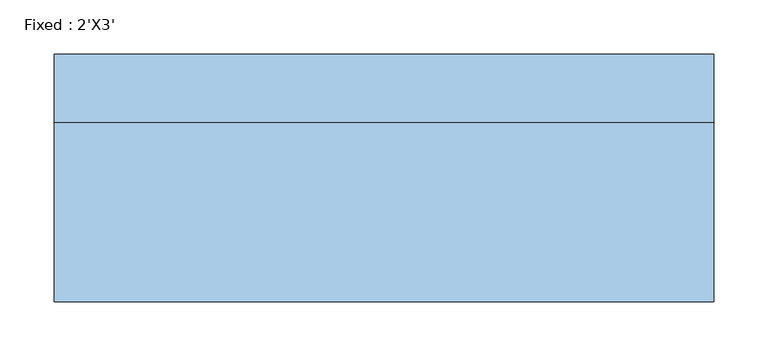
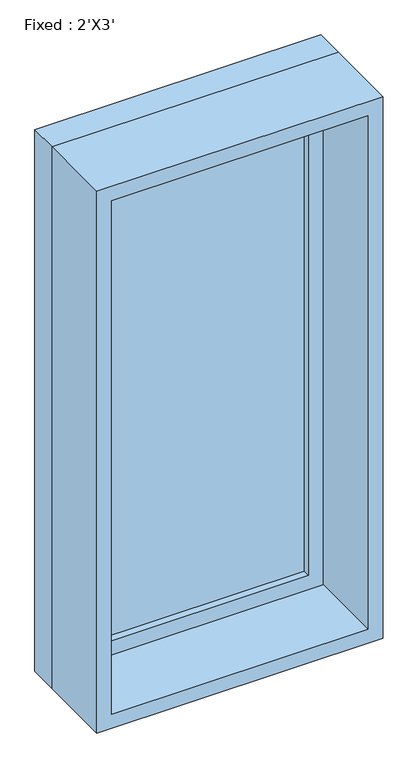
"""IFC4 building model written with IfcOpenShell, lengths in millimetres: window geometry, Fixed : 2'X3'."""

from ifc_helpers import new_model, si_unit, frame, origin, place, context, project, spatial, polyline, outline, extrude, source, transform, mapped, element, save


def fixed_2_x3_c82808a1(model_context):
    return source(origin(), model_context, "Body", "SweptSolid", [
        extrude(outline(polyline([(203.2, 66.675), (-279.4, 66.675), (-279.4, 79.375), (203.2, 79.375), (203.2, 66.675)])), frame((0.0, 0.0, 977.9), z_axis=(0.0, 0.0, 1.0), x_axis=(1.0, 0.0, 0.0)), (0.0, 0.0, 1.0), 1092.2),
        extrude(outline(polyline([(2114.55, -323.85), (933.45, -323.85), (933.45, 247.65), (2114.55, 247.65), (2114.55, -323.85)]), holes=[polyline([(2070.1, -279.4), (2070.1, 203.2), (977.9, 203.2), (977.9, -279.4), (2070.1, -279.4)])]), frame((0.0, 50.8, 0.0), z_axis=(0.0, 1.0, 0.0), x_axis=(0.0, 0.0, 1.0)), (0.0, 0.0, 1.0), 44.45),
        extrude(outline(polyline([(2133.6, -342.9), (914.4, -342.9), (914.4, 266.7), (2133.6, 266.7), (2133.6, -342.9)]), holes=[polyline([(2101.85, -311.15), (2101.85, 234.95), (946.15, 234.95), (946.15, -311.15), (2101.85, -311.15)])]), frame((0.0, -114.3, 0.0), z_axis=(0.0, 1.0, 0.0), x_axis=(0.0, 0.0, 1.0)), (0.0, 0.0, 1.0), 165.1),
        extrude(outline(polyline([(2133.6, 266.7), (2133.6, -342.9), (914.4, -342.9), (914.4, 266.7), (2133.6, 266.7)]), holes=[polyline([(2114.55, 247.65), (933.45, 247.65), (933.45, -323.85), (2114.55, -323.85), (2114.55, 247.65)])]), frame((0.0, 50.8, 0.0), z_axis=(0.0, 1.0, 0.0), x_axis=(0.0, 0.0, 1.0)), (0.0, 0.0, 1.0), 63.5),
    ])


if __name__ == "__main__":
    model = new_model("IFC4")
    model_context = context("Model", 3, world=origin())
    ifc_project = project(units=[si_unit("LENGTHUNIT", "METRE", prefix="MILLI")], contexts=[model_context])
    site = spatial("IfcSite", under=ifc_project)
    building = spatial("IfcBuilding", under=site)
    placement = place(None, origin())
    fixed_2_x3_shape = fixed_2_x3_c82808a1(model_context)
    element("IfcWindow", 1, ObjectType="Fixed : 2'X3'", at=placement, inside=building, context=model_context, shape_type="MappedRepresentation", body=[
        mapped(fixed_2_x3_shape, transform((0.0, 0.0, 0.0), x_axis=(1.0, 0.0, 0.0), y_axis=(0.0, 1.0, 0.0), z_axis=(0.0, 0.0, 1.0))),
    ])
    save(model, "model.ifc")

# Revit data of these elements
# Type "Fixed : 2'X3'"
#   Type Mark = "19"
#   Construction Type Id = "GSP4R"
#   Assembly Code = "B2020100"
#   Analytic Construction = "1/8 in Pilkington single glazing"
#   Visual Light Transmittance = 0.9
#   Solar Heat Gain Coefficient = 0.78
#   Heat Transfer Coefficient (U) = 0.6496 BTU/(h·ft²·°F)
#   Height = 4' - 0"
#   Default Sill Height = 3' - 0"
#   Width = 2' - 0"
#   Window Inset = 0' - 0 3/4"
#   Define Thermal Properties by = 1
#   Glass Pane Material = Glass
#   Sash Material = Sash
#   Wall Closure = (empty or 0)
# Element 1 (IfcWindow, "Fixed : 2'X3'")
#   Materials on its faces: "Sash", "Glass"
# Materials
#   "Glass": class "Glass", colour RGB 0 128 192, transparency 0.75, Description = "Soda Lime Glass", Cost = 0
#   "Sash": class "Wood", colour RGB 224 178 126, transparency 0, Cost = 0
